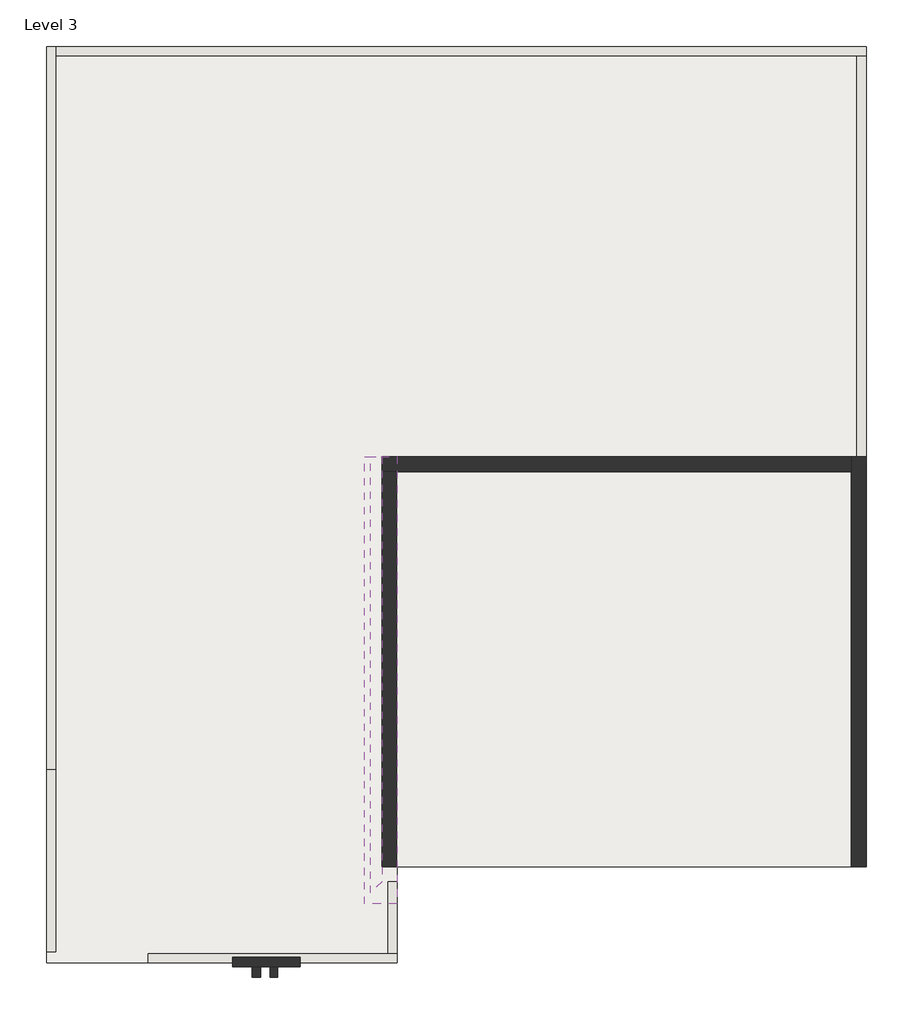
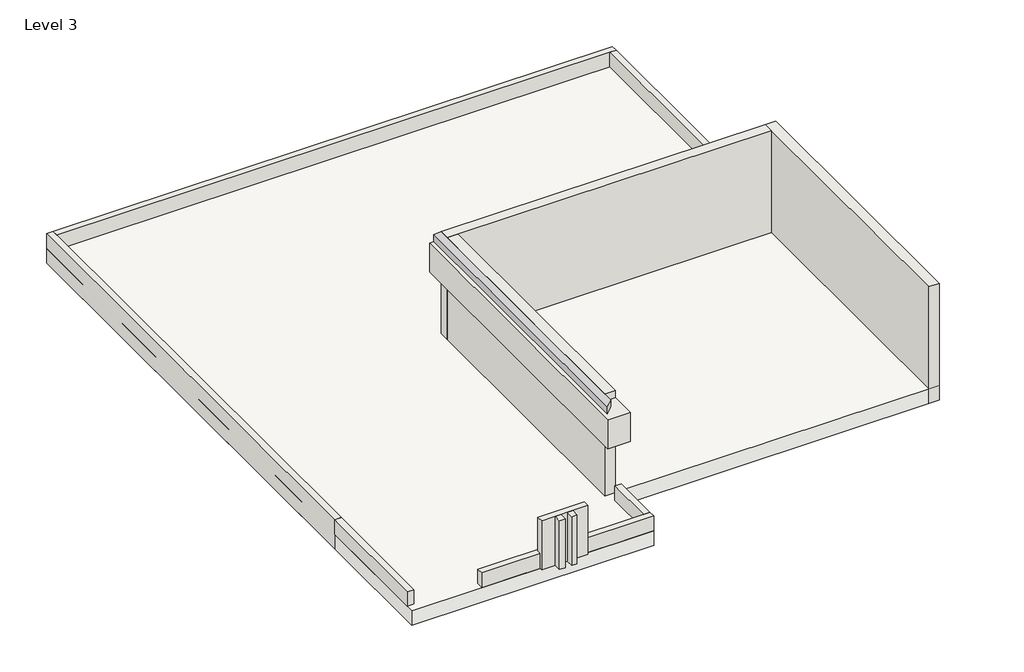
# One storey: 12 walls, 1 proxy, 1 roof.
"""IFC4 building model written with IfcOpenShell, lengths in millimetres."""

from ifc_helpers import new_model, si_unit, frame, origin, place, context, project, spatial, polyline, outline, extrude, faceted_brep, transform, mapped, element, save
from components import walls_2_walls_2_fbce2fc9, walls_3_walls_3_33d2e255

model = new_model("IFC4")

# Units and contexts
model_context = context("Model", 3, world=origin())
ifc_project = project(units=[si_unit("LENGTHUNIT", "METRE", prefix="MILLI")], contexts=[model_context])

# Site, building, storey
site = spatial("IfcSite", under=ifc_project)
building = spatial("IfcBuilding", under=site)
storey = spatial("IfcBuildingStorey", under=building, Name="Level 3", Elevation=7315.2)

# Proxy
placement = place(None, origin())
element("IfcBuildingElementProxy", 1, Name="Cornice", ObjectType="Cornice", at=placement, inside=storey, context=model_context, shape_type="SweptSolid", body=[
    extrude(outline(polyline([(-6596.5183714, 5567.8900371), (-6444.1183714, 5567.8900371), (-6444.1183714, -223.3099629), (-6596.5183714, -375.7099629), (-6596.5183714, 5567.8900371)])), frame((0.0, 0.0, 9601.2), z_axis=(0.0, 0.0, 1.0), x_axis=(1.0, 0.0, 0.0)), (0.0, 0.0, 1.0), 152.4),
])

# Roof
element("IfcRoof", 2, ObjectType="Generic - 12\"", at=placement, inside=storey, context=model_context, shape_type="SweptSolid", body=[
    extrude(outline(polyline([(-11016.1183714, 11155.8900371), (159.8816286, 11155.8900371), (159.8816286, -20.1099629), (-6234.5683714, -20.1099629), (-6234.5683714, -1332.6895946), (-11016.1183714, -1332.6895946), (-11016.1183714, 11155.8900371)])), frame((0.0, 0.0, 7315.2), z_axis=(0.0, 0.0, 1.0), x_axis=(1.0, 0.0, 0.0)), (0.0, 0.0, 1.0), 304.8),
])

# Walls
element("IfcWall", 3, ObjectType="Generic - 5\"", at=placement, inside=storey, context=model_context, shape_type="Brep", body=[
    faceted_brep([(-9633.3839949, -1332.6895946, 7620.0), (-6234.5683714, -1332.6895946, 7620.0), (-6234.5683714, -1332.6895946, 7924.8), (-9633.3839949, -1332.6895946, 7924.8), (-9633.3839949, -1205.6895946, 7620.0), (-9633.3839949, -1205.6895946, 7924.8), (-6361.5683714, -1205.6895946, 7924.8), (-6234.5683714, -1205.6895946, 7924.8), (-6234.5683714, -1205.6895946, 7620.0), (-6361.5683714, -1205.6895946, 7620.0)], [[[0, 1, 2, 3]], [[4, 5, 6, 7, 8, 9]], [[1, 0, 4, 9, 8]], [[3, 2, 7, 6, 5]], [[0, 3, 5, 4]], [[2, 1, 8, 7]]]),
])
element("IfcWall", 4, ObjectType="Generic - 5\"", at=placement, inside=storey, context=model_context, shape_type="SweptSolid", body=[
    extrude(outline(polyline([(-6234.5683714, -223.3099629), (-6234.5683714, -1205.6895946), (-6361.5683714, -1205.6895946), (-6361.5683714, -223.3099629), (-6234.5683714, -223.3099629)])), frame((0.0, 0.0, 7620.0), z_axis=(0.0, 0.0, 1.0), x_axis=(1.0, 0.0, 0.0)), (0.0, 0.0, 1.0), 304.8),
])
element("IfcWall", 5, ObjectType="Generic - 5\"", at=placement, inside=storey, context=model_context, shape_type="SweptSolid", body=[
    extrude(outline(polyline([(-11016.1183714, -1179.3008757), (-11016.1183714, 1300.6900371), (-10889.1183714, 1300.6900371), (-10889.1183714, -1179.3008757), (-11016.1183714, -1179.3008757)])), frame((0.0, 0.0, 7620.0), z_axis=(0.0, 0.0, 1.0), x_axis=(1.0, 0.0, 0.0)), (0.0, 0.0, 1.0), 304.8),
])
element("IfcWall", 6, ObjectType="Generic - 5\"", at=placement, inside=storey, context=model_context, shape_type="SweptSolid", body=[
    extrude(outline(polyline([(-7561.7183714, -1383.4895946), (-8476.1183714, -1383.4895946), (-8476.1183714, -1256.4895946), (-7561.7183714, -1256.4895946), (-7561.7183714, -1383.4895946)])), frame((0.0, 0.0, 7620.0), z_axis=(0.0, 0.0, 1.0), x_axis=(1.0, 0.0, 0.0)), (0.0, 0.0, 1.0), 1019.9265532),
])
element("IfcWall", 7, ObjectType="Generic - 5\"", at=placement, inside=storey, context=model_context, shape_type="Brep", body=[
    faceted_brep([(-11016.1183714, 11155.8900371, 7315.2), (-11016.1183714, 1300.6900371, 7315.2), (-11016.1183714, 1300.6900371, 7620.0), (-11016.1183714, 1300.6900371, 7924.8), (-11016.1183714, 11155.8900371, 7924.8), (-10889.1183714, 11155.8900371, 7315.2), (-10889.1183714, 11155.8900371, 7924.8), (-10889.1183714, 11028.8900371, 7924.8), (-10889.1183714, 1300.6900371, 7924.8), (-10889.1183714, 1300.6900371, 7620.0), (-10889.1183714, 1300.6900371, 7315.2), (-10889.1183714, 11028.8900371, 7315.2)], [[[0, 1, 2, 3, 4]], [[5, 6, 7, 8, 9, 10, 11]], [[1, 0, 5, 11, 10]], [[3, 2, 1, 10, 9, 8]], [[4, 3, 8, 7, 6]], [[0, 4, 6, 5]]]),
])
element("IfcWall", 8, ObjectType="Generic - 5\"", at=placement, inside=storey, context=model_context, shape_type="Brep", body=[
    faceted_brep([(-10889.1183714, 11028.8900371, 7315.2), (32.8816286, 11028.8900371, 7315.2), (159.8816286, 11028.8900371, 7315.2), (159.8816286, 11028.8900371, 7924.8), (32.8816286, 11028.8900371, 7924.8), (-10889.1183714, 11028.8900371, 7924.8), (-10889.1183714, 11155.8900371, 7315.2), (-10889.1183714, 11155.8900371, 7924.8), (159.8816286, 11155.8900371, 7924.8), (159.8816286, 11155.8900371, 7315.2)], [[[0, 1, 2, 3, 4, 5]], [[6, 7, 8, 9]], [[2, 1, 0, 6, 9]], [[5, 4, 3, 8, 7]], [[0, 5, 7, 6]], [[3, 2, 9, 8]]]),
])
element("IfcWall", 9, ObjectType="Generic - 5\"", at=placement, inside=storey, context=model_context, shape_type="SweptSolid", body=[
    extrude(outline(polyline([(32.8816286, 5567.8900371), (32.8816286, 11028.8900371), (159.8816286, 11028.8900371), (159.8816286, 5567.8900371), (32.8816286, 5567.8900371)])), frame((0.0, 0.0, 7315.2), z_axis=(0.0, 0.0, 1.0), x_axis=(1.0, 0.0, 0.0)), (0.0, 0.0, 1.0), 609.6),
])
element("IfcWall", 10, ObjectType="Generic - 8\"", at=placement, inside=storey, context=model_context, shape_type="Brep", body=[
    faceted_brep([(159.8816286, -20.1099629, 7315.2), (159.8816286, 5567.8900371, 7315.2), (159.8816286, 5567.8900371, 7924.8), (159.8816286, 5567.8900371, 9753.6), (159.8816286, -20.1099629, 9753.6), (-43.3183714, -20.1099629, 7315.2), (-43.3183714, -20.1099629, 9753.6), (-43.3183714, 5364.6900371, 9753.6), (-43.3183714, 5567.8900371, 9753.6), (-43.3183714, 5567.8900371, 7315.2), (-43.3183714, 5364.6900371, 7315.2), (32.8816286, 5567.8900371, 7315.2)], [[[0, 1, 2, 3, 4]], [[5, 6, 7, 8, 9, 10]], [[1, 0, 5, 10, 9, 11]], [[4, 3, 8, 7, 6]], [[0, 4, 6, 5]], [[1, 11, 9, 8, 3, 2]]]),
])
element("IfcWall", 11, ObjectType="Generic - 8\"", at=placement, inside=storey, context=model_context, shape_type="Brep", body=[
    faceted_brep([(-43.3183714, 5567.8900371, 9753.6), (-43.3183714, 5567.8900371, 7315.2), (-6444.1183714, 5567.8900371, 7315.2), (-6444.1183714, 5567.8900371, 9753.6), (-43.3183714, 5364.6900371, 7315.2), (-43.3183714, 5364.6900371, 9753.6), (-6240.9183714, 5364.6900371, 9753.6), (-6444.1183714, 5364.6900371, 9753.6), (-6444.1183714, 5364.6900371, 7315.2), (-6240.9183714, 5364.6900371, 7315.2)], [[[0, 1, 2, 3]], [[4, 5, 6, 7, 8, 9]], [[2, 1, 4, 9, 8]], [[0, 3, 7, 6, 5]], [[3, 2, 8, 7]], [[0, 5, 4, 1]]]),
])
element("IfcWall", 12, ObjectType="Generic - 8\"", at=placement, inside=storey, context=model_context, shape_type="Brep", body=[
    faceted_brep([(-6444.1183714, 5364.6900371, 7315.2), (-6444.1183714, 1199.0900371, 7315.2), (-6444.1183714, -20.1099629, 7315.2), (-6444.1183714, -20.1099629, 9601.2), (-6444.1183714, -20.1099629, 9753.6), (-6444.1183714, 5364.6900371, 9753.6), (-6444.1183714, 5364.6900371, 9601.2), (-6240.9183714, -20.1099629, 7315.2), (-6240.9183714, 1199.0900371, 7315.2), (-6240.9183714, 5364.6900371, 7315.2), (-6240.9183714, 5364.6900371, 9753.6), (-6240.9183714, -20.1099629, 9753.6)], [[[0, 1, 2, 3, 4, 5, 6]], [[7, 8, 9, 10, 11]], [[2, 1, 0, 9, 8, 7]], [[5, 4, 11, 10]], [[5, 10, 9, 0, 6]], [[2, 7, 11, 4, 3]]]),
])
walls_2_walls_2_shape = walls_2_walls_2_fbce2fc9(model_context)
element("IfcWall", 13, ObjectType="Walls 2 : Walls 2", at=placement, inside=storey, context=model_context, shape_type="MappedRepresentation", body=[
    mapped(walls_2_walls_2_shape, transform((0.0, 0.0, 0.0), x_axis=(1.0, 0.0, 0.0), y_axis=(0.0, 1.0, 0.0), z_axis=(0.0, 0.0, 1.0))),
])
walls_3_walls_3_shape = walls_3_walls_3_33d2e255(model_context)
element("IfcWall", 14, ObjectType="Walls 3 : Walls 3", at=placement, inside=storey, context=model_context, shape_type="MappedRepresentation", body=[
    mapped(walls_3_walls_3_shape, transform((0.0, 0.0, 0.0), x_axis=(1.0, 0.0, 0.0), y_axis=(0.0, 1.0, 0.0), z_axis=(0.0, 0.0, 1.0))),
])

save(model, "model.ifc")

# Revit data of these elements
# Type "Generic - 12\""
#   Assembly Code = "B1020"
#   Layers, outside or top first: 1' - 0" no material (function 1)
# Type "Generic - 5\""
#   Assembly Code = "B2010"
#   Layers, outside or top first: 0' - 5" no material (function 1)
# Type "Generic - 8\""
#   Assembly Code = "B2010"
#   Layers, outside or top first: 0' - 8" no material (function 1)
# Element 1 (IfcBuildingElementProxy, "Cornice")
#   Phase Created = New Construction
#   Materials on its faces: "Default Wall"
# Element 2 (IfcRoof, "Generic - 12\"")
#   built-in parameter 1001705 = 25 (stored number, unit not read)
#   built-in parameter 1001710 = 33615
#   Phase Created = New Construction
#   Materials on its faces: "Default Roof"
# Elements 3, 4, 5 (IfcWall, "Generic - 5\"")
#   built-in parameter 1001111 = 1' - 0"
#   Top Offset = -10' - 0"
#   Base Offset = 1' - 0"
#   wall height = 1' - 0"
#   Phase Created = New Construction
#   Base Constraint = Level 3
#   Top Constraint = Level 4
#   Materials on its faces: "Default Wall"
# Element 6 (IfcWall, "Generic - 5\"")
#   built-in parameter 1001111 = 1' - 0"
#   Top Offset = -7' - 7.84541"
#   Base Offset = 1' - 0"
#   wall height = 3' - 4.15459"
#   Phase Created = New Construction
#   Base Constraint = Level 3
#   Top Constraint = Level 4
#   Materials on its faces: "Default Wall"
# Elements 7, 8, 9 (IfcWall, "Generic - 5\"")
#   Top Offset = -10' - 0"
#   Base Offset = 0' - 0"
#   wall height = 2' - 0"
#   Phase Created = New Construction
#   Base Constraint = Level 3
#   Top Constraint = Level 4
#   Materials on its faces: "Default Wall"
# Elements 10, 11, 12 (IfcWall, "Generic - 8\"")
#   Top Offset = 0' - 0"
#   Base Offset = 0' - 0"
#   Unconnected Height = 8' - 0"
#   wall height = 8' - 0"
#   Phase Created = New Construction
#   Base Constraint = Level 3
#   Materials on its faces: "Default Wall"
# Element 13 (IfcWall, "Walls 2 : Walls 2")
#   Phase Created = New Construction
#   Materials on its faces: "Default Wall"
# Element 14 (IfcWall, "Walls 3 : Walls 3")
#   Phase Created = New Construction
#   Materials on its faces: "Default Wall"
# Materials
#   "Default Wall": colour RGB 128 128 128, transparency 0
#   "Default Roof": colour RGB 88 101 114, transparency 0
